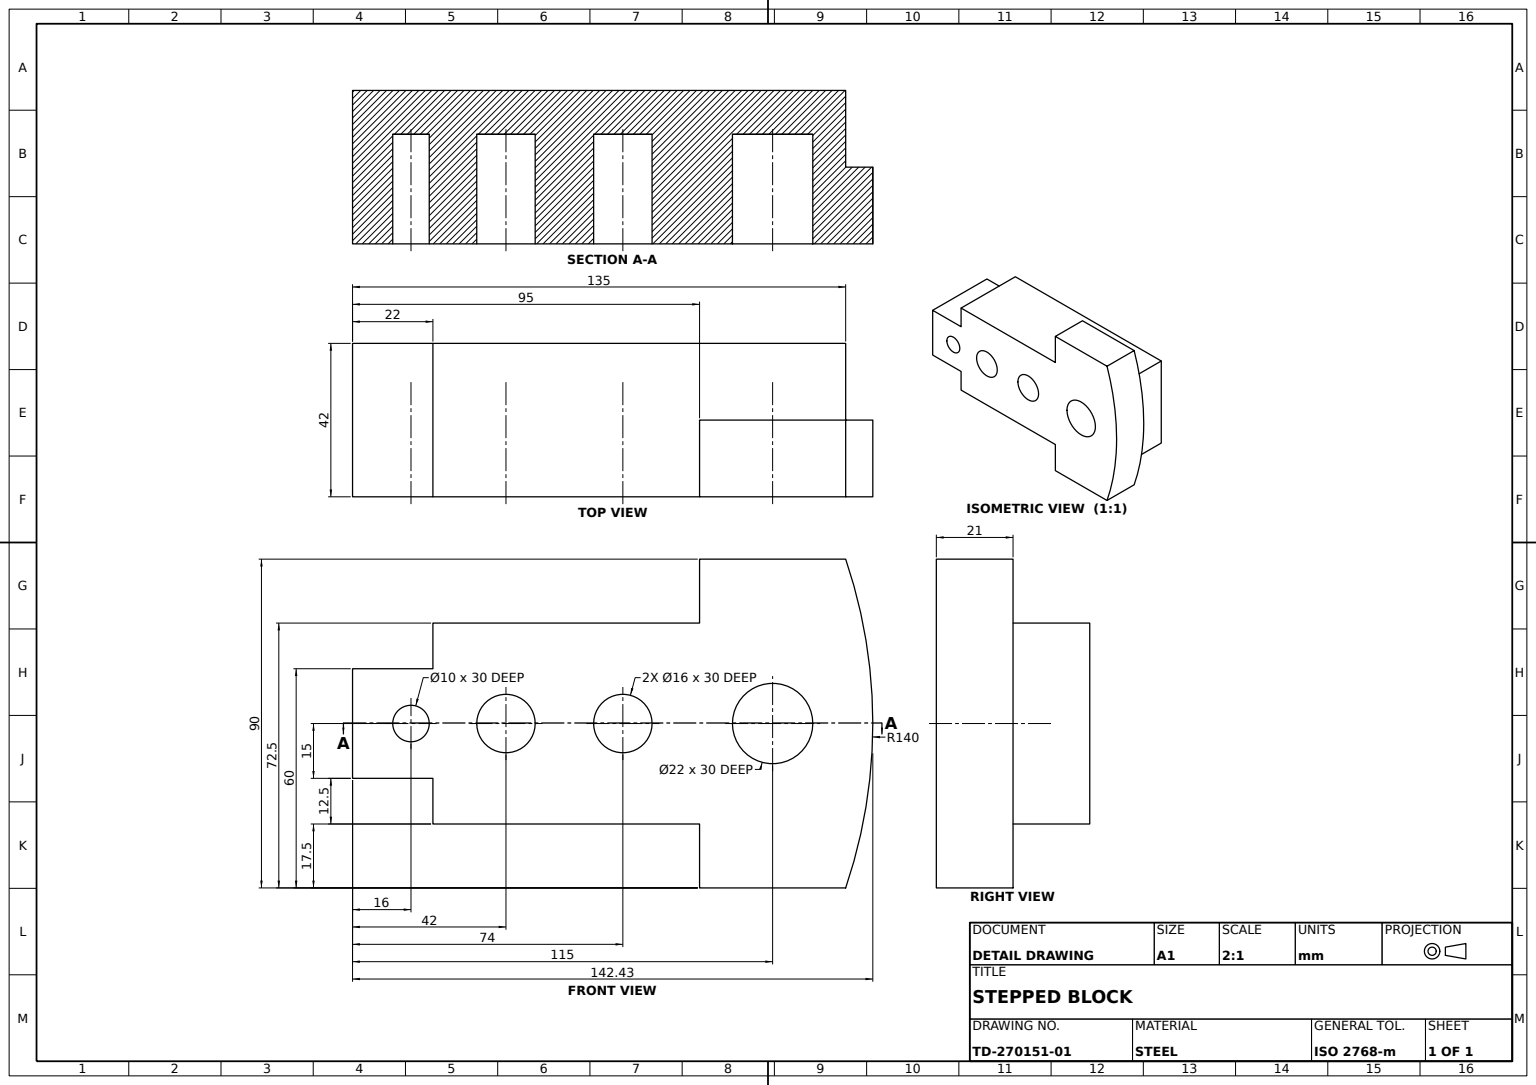
from build123d import *

# Parameters (mm, degrees)
BASE_BLOCK_63MM_DEPTH      = 63
PROFILE_CUT_63MM_DEPTH     = 63
SIDE_BOSS_SKETCH_W         = 63
SIDE_BOSS_SKETCH_H         = 90
SIDE_BOSS_16MM_DEPTH       = 16
STEP_CUT_21MM_DEPTH        = 21
CURVED_END_BOSS_21MM_DEPTH = 21
POCKET_CUT_SKETCH_W        = 21
POCKET_CUT_SKETCH_H        = 17.5
POCKET_CUT_40MM_DEPTH      = 40
HOLE_A_SKETCH_W            = 73
HOLE_A_SKETCH_H            = 42
HOLE_A_17_5MM_DEEP_DEPTH   = 17.5
HOLE_B_SKETCH_W            = 73
HOLE_B_SKETCH_H            = 42
HOLE_B_17_5MM_DEEP_DEPTH   = 17.5
END_CUT_SKETCH_R           = 11
END_CUT_SKETCH_R_2         = 8
END_CUT_SKETCH_R_3         = 5
END_CUT_30MM_DEPTH         = 30


with BuildPart() as part:
    # Base Profile Sketch → Base Block 63mm (new body)
    with BuildSketch(Plane.XY):
        Polygon((0, 0), (115, 0), (115, 90), (54, 90), (22, 90), (-4, 90), (-4, 0), align=None)
    extrude(amount=BASE_BLOCK_63MM_DEPTH)

    # Profile Cut Sketch → Profile Cut 63mm (cut)
    with BuildSketch(Plane.XY.offset(63)):
        Polygon((18, 60), (18, 72.5), (18, 90), (-4, 90), (-4, 72.5), (-4, 60), align=None)
        Polygon((18, 30), (-4, 30), (-4, 17.5), (-4, 0), (18, 0), (18, 17.5), align=None)
    extrude(amount=-PROFILE_CUT_63MM_DEPTH, mode=Mode.SUBTRACT)

    # Side Boss Sketch → Side Boss 16mm (add)
    with BuildSketch(Plane(origin=(115, 0, 0), x_dir=(0, 0, -1), z_dir=(1, 0, 0))):
        with Locations((-31.5, 45)):
            Rectangle(SIDE_BOSS_SKETCH_W, SIDE_BOSS_SKETCH_H)
    extrude(amount=SIDE_BOSS_16MM_DEPTH)

    # Step Cut Sketch → Step Cut 21mm (cut)
    with BuildSketch(Plane.XY.offset(63)):
        Polygon((18, 90), (91, 90), (131, 90), (131, 0), (91, 0), (18, 0), (18, 30), (-4, 30), (-4, 60), (18, 60), align=None)
    extrude(amount=-STEP_CUT_21MM_DEPTH, mode=Mode.SUBTRACT)

    # Curved End Boss Sketch → Curved End Boss 21mm (add)
    with BuildSketch(Plane.XY.offset(42)):
        with BuildLine():
            Line((131, 90), (131, 0))
            ThreePointArc((131, 0), (138.429264164, 45), (131, 90))
        make_face()
    extrude(amount=-CURVED_END_BOSS_21MM_DEPTH)

    # Pocket Cut Sketch → Pocket Cut 40mm (cut)
    with BuildSketch(Plane(origin=(131, 0, 0), x_dir=(0, 0, -1), z_dir=(1, 0, 0))):
        with Locations((-10.5, 81.25)):
            Rectangle(POCKET_CUT_SKETCH_W, POCKET_CUT_SKETCH_H)
        with Locations((-10.5, 8.75)):
            Rectangle(POCKET_CUT_SKETCH_W, POCKET_CUT_SKETCH_H)
    extrude(amount=-POCKET_CUT_40MM_DEPTH, mode=Mode.SUBTRACT)

    # Hole A Sketch → Hole A 17.5mm Deep (cut)
    with BuildSketch(Plane.XZ):
        with Locations((54.5, 21)):
            Rectangle(HOLE_A_SKETCH_W, HOLE_A_SKETCH_H)
    extrude(amount=-HOLE_A_17_5MM_DEEP_DEPTH, mode=Mode.SUBTRACT)

    # Hole B Sketch → Hole B 17.5mm Deep (cut)
    with BuildSketch(Plane(origin=(0, 90, 0), x_dir=(1, 0, 0), z_dir=(0, 1, 0))):
        with Locations((54.5, -21)):
            Rectangle(HOLE_B_SKETCH_W, HOLE_B_SKETCH_H)
    extrude(amount=-HOLE_B_17_5MM_DEEP_DEPTH, mode=Mode.SUBTRACT)

    # End Cut Sketch → End Cut 30mm (cut)
    with BuildSketch(Plane.XY.offset(42)):
        with Locations((111, 45)):
            Circle(END_CUT_SKETCH_R)
        with Locations((70, 45)):
            Circle(END_CUT_SKETCH_R_2)
        with Locations((38, 45)):
            Circle(END_CUT_SKETCH_R_2)
        with Locations((12, 45)):
            Circle(END_CUT_SKETCH_R_3)
    extrude(amount=-END_CUT_30MM_DEPTH, mode=Mode.SUBTRACT)


solid = part.part
